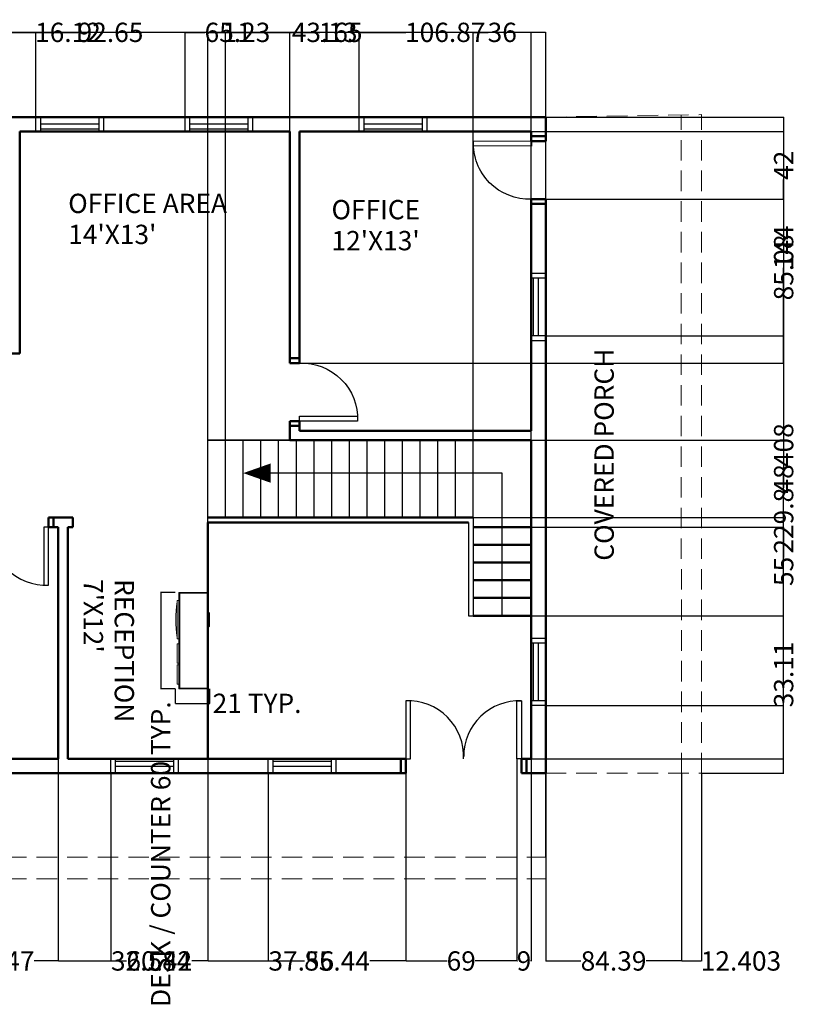
# Model space of a CAD drawing. Units: inches. Extents: x 128 to 1267, y -109 to 1208.
# Tile 4 of 8: x 784 to 1267, y -109 to 503. Entities that reach past the tile are written whole.
import ezdxf

# ---------------------------------------------------------------- set-up
doc = ezdxf.new("R2010")
doc.units = ezdxf.units.IN
doc.header["$MEASUREMENT"] = 0
doc.linetypes.add('DASHED', pattern=[19.05, 12.7, -6.35])
for name, color, linetype, lineweight in [('A-ANNO-DIMS', 2, 'Continuous', 18), ('A-AREA-IDEN', 3, 'Continuous', 25), ('A-DOOR', 4, 'Continuous', 25), ('A-FLOR-STRS', 2, 'Continuous', 25), ('A-FURN', 8, 'Continuous', 18), ('A-GLAZ', 3, 'Continuous', 25), ('A-ROOF-OVHD', 9, 'DASHED', 18), ('A-WALL', 7, 'Continuous', 50)]:
    doc.layers.add(name, color=color, linetype=linetype, lineweight=lineweight)
doc.styles.get("Standard").update_dxf_attribs({"font": 'arial.ttf'})
doc.dimstyles.get("Standard").update_dxf_attribs({"dimtxt": 12, "dimasz": 0.18, "dimexe": 0.18, "dimexo": 0.0625, "dimgap": 0.09, "dimtad": 0, "dimdec": 1, "dimzin": 0, "dimdsep": 46, "dimlunit": 3, "dimtxsty": 'Standard', "dimcen": 0.09, "dimadec": 0, "dimazin": 0, "dimtfac": 1, "dimtdec": 1, "dimtofl": 0, "dimtmove": 0, "dimatfit": 3, "dimfxl": 1, "dimtolj": 1, "dimtzin": 0, "dimarcsym": 0})

# ---------------------------------------------------------------- blocks, each defined once
blk = doc.blocks.new('Entertainment Center')
for p, q in [((-4, 0), (-5, -1)), ((4, 0), (-4, 0)), ((5, -1), (4, 0)), ((-17, -19), (-17, -1)), ((-17, -1), (43, -1)), ((-16.5, -18.5), (-16.5, -1.5)), ((-16.5, -1.5), (42.5, -1.5)), ((42.5, -1.5), (42.5, -18.5)), ((43, -1), (43, -19)), ((43, -19), (-17, -19)), ((42.5, -18.5), (-16.5, -18.5)), ((-12, -20), (-12, -19)), ((12, -20), (-12, -20)), ((12, -19), (12, -20)), ((15, -20), (15, -19)), ((27, -20), (15, -20)), ((27, -19), (27, -20)), ((28, -20), (28, -19)), ((40, -20), (28, -20)), ((40, -19), (40, -20))]:
    blk.add_line(p, q)
blk.add_arc((0, 40), 61, 259.6111, 280.3889)
blk = doc.blocks.new('DOOR-900')
blk.add_lwpolyline([(460.06, 187.64), (457.06, 187.64), (457.06, 151.64), (460.06, 151.64)], close=True)
blk.add_arc((458.56, 186.14), 34.53, 177.51045, 272.48955)
blk = doc.blocks.new('WIN-900')
for p, q in [((1102.06, 345.56), (1111.06, 345.56)), ((1102.06, 342.56), (1111.06, 342.56)), ((1103.56, 306.56), (1103.56, 342.56)), ((1106.56, 306.56), (1106.56, 342.56)), ((1111.06, 306.56), (1102.06, 306.56)), ((1111.06, 303.56), (1102.06, 303.56))]:
    blk.add_line(p, q)
blk = doc.blocks.new('*D12')
at = {"layer": 'A-ANNO-DIMS', "color": 0, "lineweight": -2, "transparency": 16777216}
for p, q in [((880.66, 147.14), (871.54, 147.14)), ((871.72, 146.96), (871.72, 87.32)), ((880.66, 87.14), (871.54, 87.14)), ((871.72, 87.14), (871.72, 86.96))]:
    blk.add_line(p, q, dxfattribs=at)
at = {"layer": 'A-ANNO-DIMS', "color": 0, "transparency": 16777216}
for points in [[(871.69, 146.96), (871.75, 146.96), (871.72, 147.14)], [(871.69, 87.32), (871.75, 87.32), (871.72, 87.14)]]:
    blk.add_solid(points, dxfattribs=at)
at = {"layer": 'Defpoints', "color": 0, "transparency": 16777216}
for p in [(880.72, 147.14), (871.72, 87.14), (880.72, 87.14)]:
    blk.add_point(p, dxfattribs=at)
at = {"layer": 'A-ANNO-DIMS', "color": 0, "transparency": 16777216, "insert": (871.72, -15.62), "char_height": 12, "attachment_point": 5, "rotation": 90}
blk.add_mtext('\\A1;DESK / COUNTER 60 TYP.', dxfattribs=at)
blk = doc.blocks.new('*D13')
at = {"layer": 'A-ANNO-DIMS', "color": 0, "lineweight": -2, "transparency": 16777216}
for p, q in [((880.72, 87.08), (880.72, 77.96)), ((902.06, 87.08), (902.06, 77.96)), ((880.9, 78.14), (901.88, 78.14)), ((902.06, 78.14), (902.24, 78.14))]:
    blk.add_line(p, q, dxfattribs=at)
at = {"layer": 'A-ANNO-DIMS', "color": 0, "transparency": 16777216}
for points in [[(880.9, 78.17), (880.9, 78.11), (880.72, 78.14)], [(901.88, 78.17), (901.88, 78.11), (902.06, 78.14)]]:
    blk.add_solid(points, dxfattribs=at)
at = {"layer": 'Defpoints', "color": 0, "transparency": 16777216}
for p in [(880.72, 87.14), (902.06, 87.14), (902.06, 78.14)]:
    blk.add_point(p, dxfattribs=at)
at = {"layer": 'A-ANNO-DIMS', "color": 0, "transparency": 16777216, "insert": (931.63, 78.14), "char_height": 12, "attachment_point": 5}
blk.add_mtext('\\A1;21 TYP.', dxfattribs=at)
blk = doc.blocks.new('*D22')
at = {"layer": 'A-ANNO-DIMS', "color": 0, "lineweight": -2, "transparency": 16777216}
for p, q in [((223.06, -17.52), (223.06, 495.44)), ((223.24, 495.26), (653.69, 495.26)), ((1110.88, 495.26), (680.42, 495.26)), ((1111.06, -17.52), (1111.06, 495.44))]:
    blk.add_line(p, q, dxfattribs=at)
at = {"layer": 'A-ANNO-DIMS', "color": 0, "transparency": 16777216}
for points in [[(223.24, 495.29), (223.24, 495.23), (223.06, 495.26)], [(1110.88, 495.29), (1110.88, 495.23), (1111.06, 495.26)]]:
    blk.add_solid(points, dxfattribs=at)
at = {"layer": 'Defpoints', "color": 0, "transparency": 16777216}
for p in [(1111.06, 495.26), (223.06, -17.58), (1111.06, -17.58)]:
    blk.add_point(p, dxfattribs=at)
at = {"layer": 'A-ANNO-DIMS', "color": 0, "transparency": 16777216, "insert": (667.06, 495.26), "char_height": 12, "attachment_point": 5}
blk.add_mtext('\\A1;888', dxfattribs=at)
blk = doc.blocks.new('*D23')
at = {"layer": 'A-ANNO-DIMS', "color": 0, "lineweight": -2, "transparency": 16777216}
for p, q in [((1111.12, 442.64), (1259.18, 442.64)), ((1259, 442.46), (1259, 252.24)), ((1259, 34.82), (1259, 225.04)), ((1207.91, 34.64), (1259.18, 34.64))]:
    blk.add_line(p, q, dxfattribs=at)
at = {"layer": 'A-ANNO-DIMS', "color": 0, "transparency": 16777216}
for points in [[(1258.97, 442.46), (1259.03, 442.46), (1259, 442.64)], [(1258.97, 34.82), (1259.03, 34.82), (1259, 34.64)]]:
    blk.add_solid(points, dxfattribs=at)
at = {"layer": 'Defpoints', "color": 0, "transparency": 16777216}
for p in [(1111.06, 442.64), (1207.85, 34.64), (1259, 34.64)]:
    blk.add_point(p, dxfattribs=at)
at = {"layer": 'A-ANNO-DIMS', "color": 0, "transparency": 16777216, "insert": (1259, 238.64), "char_height": 12, "attachment_point": 5, "rotation": 90}
blk.add_mtext('\\A1;408', dxfattribs=at)
blk = doc.blocks.new('*D24')
at = {"layer": 'A-ANNO-DIMS', "color": 0, "lineweight": -2, "transparency": 16777216}
for p, q in [((1111.06, 34.58), (1111.06, -82.19)), ((1195.45, 34.58), (1195.45, -82.19)), ((1111.24, -82.01), (1132.89, -82.01)), ((1195.27, -82.01), (1173.61, -82.01))]:
    blk.add_line(p, q, dxfattribs=at)
at = {"layer": 'A-ANNO-DIMS', "color": 0, "transparency": 16777216}
for points in [[(1111.24, -81.98), (1111.24, -82.04), (1111.06, -82.01)], [(1195.27, -81.98), (1195.27, -82.04), (1195.45, -82.01)]]:
    blk.add_solid(points, dxfattribs=at)
at = {"layer": 'Defpoints', "color": 0, "transparency": 16777216}
for p in [(1111.06, 34.64), (1195.45, 34.64), (1195.45, -82.01)]:
    blk.add_point(p, dxfattribs=at)
at = {"layer": 'A-ANNO-DIMS', "color": 0, "transparency": 16777216, "insert": (1153.25, -82.01), "char_height": 12, "attachment_point": 5}
blk.add_mtext('\\A1;84.39', dxfattribs=at)
blk = doc.blocks.new('*D25')
at = {"layer": 'A-ANNO-DIMS', "color": 0, "lineweight": -2, "transparency": 16777216}
for p, q in [((1195.45, 34.58), (1195.45, -82.19)), ((1207.85, 34.58), (1207.85, -82.19)), ((1195.63, -82.01), (1207.67, -82.01)), ((1207.85, -82.01), (1208.03, -82.01))]:
    blk.add_line(p, q, dxfattribs=at)
at = {"layer": 'A-ANNO-DIMS', "color": 0, "transparency": 16777216}
for points in [[(1195.63, -81.98), (1195.63, -82.04), (1195.45, -82.01)], [(1207.67, -81.98), (1207.67, -82.04), (1207.85, -82.01)]]:
    blk.add_solid(points, dxfattribs=at)
at = {"layer": 'Defpoints', "color": 0, "transparency": 16777216}
for p in [(1195.45, 34.64), (1207.85, 34.64), (1207.85, -82.01)]:
    blk.add_point(p, dxfattribs=at)
at = {"layer": 'A-ANNO-DIMS', "color": 0, "transparency": 16777216, "insert": (1232.46, -82.01), "char_height": 12, "attachment_point": 5}
blk.add_mtext('\\A1;12.403', dxfattribs=at)
blk = doc.blocks.new('*D35')
at = {"layer": 'A-ANNO-DIMS', "color": 0, "lineweight": -2, "transparency": 16777216}
for p, q in [((808.06, 43.58), (808.06, -82.19)), ((737.59, 34.58), (737.59, -82.19)), ((737.77, -82.01), (752.54, -82.01)), ((807.88, -82.01), (793.11, -82.01))]:
    blk.add_line(p, q, dxfattribs=at)
at = {"layer": 'A-ANNO-DIMS', "color": 0, "transparency": 16777216}
for points in [[(737.77, -81.98), (737.77, -82.04), (737.59, -82.01)], [(807.88, -81.98), (807.88, -82.04), (808.06, -82.01)]]:
    blk.add_solid(points, dxfattribs=at)
at = {"layer": 'Defpoints', "color": 0, "transparency": 16777216}
for p in [(808.06, 43.64), (737.59, 34.64), (808.06, -82.01)]:
    blk.add_point(p, dxfattribs=at)
at = {"layer": 'A-ANNO-DIMS', "color": 0, "transparency": 16777216, "insert": (772.82, -82.01), "char_height": 12, "attachment_point": 5}
blk.add_mtext('\\A1;70.47', dxfattribs=at)
blk = doc.blocks.new('*D36')
at = {"layer": 'A-ANNO-DIMS', "color": 0, "lineweight": -2, "transparency": 16777216}
for p, q in [((808.06, 43.58), (808.06, -82.19)), ((840.64, 34.58), (840.64, -82.19)), ((808.24, -82.01), (840.46, -82.01)), ((840.64, -82.01), (840.82, -82.01))]:
    blk.add_line(p, q, dxfattribs=at)
at = {"layer": 'A-ANNO-DIMS', "color": 0, "transparency": 16777216}
for points in [[(808.24, -81.98), (808.24, -82.04), (808.06, -82.01)], [(840.46, -81.98), (840.46, -82.04), (840.64, -82.01)]]:
    blk.add_solid(points, dxfattribs=at)
at = {"layer": 'Defpoints', "color": 0, "transparency": 16777216}
for p in [(808.06, 43.64), (840.64, 34.64), (840.64, -82.01)]:
    blk.add_point(p, dxfattribs=at)
at = {"layer": 'A-ANNO-DIMS', "color": 0, "transparency": 16777216, "insert": (865.79, -82.01), "char_height": 12, "attachment_point": 5}
blk.add_mtext('\\A1;32.584', dxfattribs=at)
blk = doc.blocks.new('*D37')
at = {"layer": 'A-ANNO-DIMS', "color": 0, "lineweight": -2, "transparency": 16777216}
for p, q in [((901.06, 43.58), (901.06, -82.19)), ((840.64, 34.58), (840.64, -82.19)), ((840.82, -82.01), (850.54, -82.01)), ((900.88, -82.01), (891.16, -82.01))]:
    blk.add_line(p, q, dxfattribs=at)
at = {"layer": 'A-ANNO-DIMS', "color": 0, "transparency": 16777216}
for points in [[(840.82, -81.98), (840.82, -82.04), (840.64, -82.01)], [(900.88, -81.98), (900.88, -82.04), (901.06, -82.01)]]:
    blk.add_solid(points, dxfattribs=at)
at = {"layer": 'Defpoints', "color": 0, "transparency": 16777216}
for p in [(901.06, 43.64), (840.64, 34.64), (901.06, -82.01)]:
    blk.add_point(p, dxfattribs=at)
at = {"layer": 'A-ANNO-DIMS', "color": 0, "transparency": 16777216, "insert": (870.85, -82.01), "char_height": 12, "attachment_point": 5}
blk.add_mtext('\\A1;60.42', dxfattribs=at)
blk = doc.blocks.new('*D38')
at = {"layer": 'A-ANNO-DIMS', "color": 0, "lineweight": -2, "transparency": 16777216}
for p, q in [((901.06, 43.58), (901.06, -82.19)), ((938.62, 34.58), (938.62, -82.19)), ((901.24, -82.01), (938.44, -82.01)), ((938.62, -82.01), (938.8, -82.01))]:
    blk.add_line(p, q, dxfattribs=at)
at = {"layer": 'A-ANNO-DIMS', "color": 0, "transparency": 16777216}
for points in [[(901.24, -81.98), (901.24, -82.04), (901.06, -82.01)], [(938.44, -81.98), (938.44, -82.04), (938.62, -82.01)]]:
    blk.add_solid(points, dxfattribs=at)
at = {"layer": 'Defpoints', "color": 0, "transparency": 16777216}
for p in [(901.06, 43.64), (938.62, 34.64), (938.62, -82.01)]:
    blk.add_point(p, dxfattribs=at)
at = {"layer": 'A-ANNO-DIMS', "color": 0, "transparency": 16777216, "insert": (959.13, -82.01), "char_height": 12, "attachment_point": 5}
blk.add_mtext('\\A1;37.56', dxfattribs=at)
blk = doc.blocks.new('*D39')
at = {"layer": 'A-ANNO-DIMS', "color": 0, "lineweight": -2, "transparency": 16777216}
for p, q in [((938.62, 34.58), (938.62, -82.19)), ((1024.06, 34.58), (1024.06, -82.19)), ((938.8, -82.01), (961.02, -82.01)), ((1023.88, -82.01), (1001.66, -82.01))]:
    blk.add_line(p, q, dxfattribs=at)
at = {"layer": 'A-ANNO-DIMS', "color": 0, "transparency": 16777216}
for points in [[(938.8, -81.98), (938.8, -82.04), (938.62, -82.01)], [(1023.88, -81.98), (1023.88, -82.04), (1024.06, -82.01)]]:
    blk.add_solid(points, dxfattribs=at)
at = {"layer": 'Defpoints', "color": 0, "transparency": 16777216}
for p in [(938.62, 34.64), (1024.06, 34.64), (1024.06, -82.01)]:
    blk.add_point(p, dxfattribs=at)
at = {"layer": 'A-ANNO-DIMS', "color": 0, "transparency": 16777216, "insert": (981.34, -82.01), "char_height": 12, "attachment_point": 5}
blk.add_mtext('\\A1;85.44', dxfattribs=at)
blk = doc.blocks.new('*D40')
at = {"layer": 'A-ANNO-DIMS', "color": 0, "lineweight": -2, "transparency": 16777216}
for p, q in [((1093.06, 43.58), (1093.06, -82.19)), ((1024.06, 34.58), (1024.06, -82.19)), ((1024.24, -82.01), (1049.83, -82.01)), ((1092.88, -82.01), (1067.29, -82.01))]:
    blk.add_line(p, q, dxfattribs=at)
at = {"layer": 'A-ANNO-DIMS', "color": 0, "transparency": 16777216}
for points in [[(1024.24, -81.98), (1024.24, -82.04), (1024.06, -82.01)], [(1092.88, -81.98), (1092.88, -82.04), (1093.06, -82.01)]]:
    blk.add_solid(points, dxfattribs=at)
at = {"layer": 'Defpoints', "color": 0, "transparency": 16777216}
for p in [(1093.06, 43.64), (1024.06, 34.64), (1093.06, -82.01)]:
    blk.add_point(p, dxfattribs=at)
at = {"layer": 'A-ANNO-DIMS', "color": 0, "transparency": 16777216, "insert": (1058.56, -82.01), "char_height": 12, "attachment_point": 5}
blk.add_mtext('\\A1;69', dxfattribs=at)
blk = doc.blocks.new('*D41')
at = {"layer": 'A-ANNO-DIMS', "color": 0, "lineweight": -2, "transparency": 16777216}
for p, q in [((1093.06, 43.58), (1093.06, -82.19)), ((1102.06, 43.58), (1102.06, -82.19)), ((1093.24, -82.01), (1093.52, -82.01)), ((1101.88, -82.01), (1101.59, -82.01))]:
    blk.add_line(p, q, dxfattribs=at)
at = {"layer": 'A-ANNO-DIMS', "color": 0, "transparency": 16777216}
for points in [[(1093.24, -81.98), (1093.24, -82.04), (1093.06, -82.01)], [(1101.88, -81.98), (1101.88, -82.04), (1102.06, -82.01)]]:
    blk.add_solid(points, dxfattribs=at)
at = {"layer": 'Defpoints', "color": 0, "transparency": 16777216}
for p in [(1093.06, 43.64), (1102.06, 43.64), (1102.06, -82.01)]:
    blk.add_point(p, dxfattribs=at)
at = {"layer": 'A-ANNO-DIMS', "color": 0, "transparency": 16777216, "insert": (1097.56, -82.01), "char_height": 12, "attachment_point": 5}
blk.add_mtext('\\A1;9', dxfattribs=at)
blk = doc.blocks.new('*D51')
at = {"layer": 'A-ANNO-DIMS', "color": 0, "lineweight": -2, "transparency": 16777216}
for p, q in [((778.06, 433.7), (778.06, 495.44)), ((778.24, 495.26), (794, 495.26)), ((794.18, 442.7), (794.18, 495.44)), ((794.18, 495.26), (794.36, 495.26))]:
    blk.add_line(p, q, dxfattribs=at)
at = {"layer": 'A-ANNO-DIMS', "color": 0, "transparency": 16777216}
for points in [[(778.24, 495.29), (778.24, 495.23), (778.06, 495.26)], [(794, 495.29), (794, 495.23), (794.18, 495.26)]]:
    blk.add_solid(points, dxfattribs=at)
at = {"layer": 'Defpoints', "color": 0, "transparency": 16777216}
for p in [(794.18, 495.26), (794.18, 442.64), (778.06, 433.64)]:
    blk.add_point(p, dxfattribs=at)
at = {"layer": 'A-ANNO-DIMS', "color": 0, "transparency": 16777216, "insert": (814.07, 495.26), "char_height": 12, "attachment_point": 5}
blk.add_mtext('\\A1;16.12', dxfattribs=at)
blk = doc.blocks.new('*D52')
at = {"layer": 'A-ANNO-DIMS', "color": 0, "lineweight": -2, "transparency": 16777216}
for p, q in [((794.18, 442.7), (794.18, 495.44)), ((794.36, 495.26), (820.12, 495.26)), ((886.65, 495.26), (860.88, 495.26)), ((886.83, 442.7), (886.83, 495.44))]:
    blk.add_line(p, q, dxfattribs=at)
at = {"layer": 'A-ANNO-DIMS', "color": 0, "transparency": 16777216}
for points in [[(794.36, 495.29), (794.36, 495.23), (794.18, 495.26)], [(886.65, 495.29), (886.65, 495.23), (886.83, 495.26)]]:
    blk.add_solid(points, dxfattribs=at)
at = {"layer": 'Defpoints', "color": 0, "transparency": 16777216}
for p in [(886.83, 495.26), (794.18, 442.64), (886.83, 442.64)]:
    blk.add_point(p, dxfattribs=at)
at = {"layer": 'A-ANNO-DIMS', "color": 0, "transparency": 16777216, "insert": (840.5, 495.26), "char_height": 12, "attachment_point": 5}
blk.add_mtext('\\A1;92.65', dxfattribs=at)
blk = doc.blocks.new('*D53')
at = {"layer": 'A-ANNO-DIMS', "color": 0, "lineweight": -2, "transparency": 16777216}
for p, q in [((886.83, 442.7), (886.83, 495.44)), ((887.01, 495.26), (899.07, 495.26)), ((951.88, 495.26), (939.81, 495.26)), ((952.06, 433.7), (952.06, 495.44))]:
    blk.add_line(p, q, dxfattribs=at)
at = {"layer": 'A-ANNO-DIMS', "color": 0, "transparency": 16777216}
for points in [[(887.01, 495.29), (887.01, 495.23), (886.83, 495.26)], [(951.88, 495.29), (951.88, 495.23), (952.06, 495.26)]]:
    blk.add_solid(points, dxfattribs=at)
at = {"layer": 'Defpoints', "color": 0, "transparency": 16777216}
for p in [(952.06, 495.26), (886.83, 442.64), (952.06, 433.64)]:
    blk.add_point(p, dxfattribs=at)
at = {"layer": 'A-ANNO-DIMS', "color": 0, "transparency": 16777216, "insert": (919.44, 495.26), "char_height": 12, "attachment_point": 5}
blk.add_mtext('\\A1;65.23', dxfattribs=at)
blk = doc.blocks.new('*D54')
at = {"layer": 'A-ANNO-DIMS', "color": 0, "lineweight": -2, "transparency": 16777216}
for p, q in [((952.06, 433.7), (952.06, 495.44)), ((952.24, 495.26), (953.04, 495.26)), ((995, 495.26), (994.2, 495.26)), ((995.18, 442.7), (995.18, 495.44))]:
    blk.add_line(p, q, dxfattribs=at)
at = {"layer": 'A-ANNO-DIMS', "color": 0, "transparency": 16777216}
for points in [[(952.24, 495.29), (952.24, 495.23), (952.06, 495.26)], [(995, 495.29), (995, 495.23), (995.18, 495.26)]]:
    blk.add_solid(points, dxfattribs=at)
at = {"layer": 'Defpoints', "color": 0, "transparency": 16777216}
for p in [(995.18, 495.26), (995.18, 442.64), (952.06, 433.64)]:
    blk.add_point(p, dxfattribs=at)
at = {"layer": 'A-ANNO-DIMS', "color": 0, "transparency": 16777216, "insert": (973.62, 495.26), "char_height": 12, "attachment_point": 5}
blk.add_mtext('\\A1;43.13', dxfattribs=at)
blk = doc.blocks.new('*D55')
at = {"layer": 'A-ANNO-DIMS', "color": 0, "lineweight": -2, "transparency": 16777216}
for p, q in [((995.18, 442.7), (995.18, 495.44)), ((995.36, 495.26), (1024.19, 495.26)), ((1101.88, 495.26), (1073.05, 495.26)), ((1102.06, 433.7), (1102.06, 495.44))]:
    blk.add_line(p, q, dxfattribs=at)
at = {"layer": 'A-ANNO-DIMS', "color": 0, "transparency": 16777216}
for points in [[(995.36, 495.29), (995.36, 495.23), (995.18, 495.26)], [(1101.88, 495.29), (1101.88, 495.23), (1102.06, 495.26)]]:
    blk.add_solid(points, dxfattribs=at)
at = {"layer": 'Defpoints', "color": 0, "transparency": 16777216}
for p in [(1102.06, 495.26), (995.18, 442.64), (1102.06, 433.64)]:
    blk.add_point(p, dxfattribs=at)
at = {"layer": 'A-ANNO-DIMS', "color": 0, "transparency": 16777216, "insert": (1048.62, 495.26), "char_height": 12, "attachment_point": 5}
blk.add_mtext('\\A1;106.87', dxfattribs=at)
blk = doc.blocks.new('*D60')
at = {"layer": 'A-ANNO-DIMS', "color": 0, "lineweight": -2, "transparency": 16777216}
for p, q in [((1111.12, 76.75), (1259.18, 76.75)), ((1259, 76.75), (1259, 76.93)), ((1259, 43.82), (1259, 76.57)), ((1102.12, 43.64), (1259.18, 43.64))]:
    blk.add_line(p, q, dxfattribs=at)
at = {"layer": 'A-ANNO-DIMS', "color": 0, "transparency": 16777216}
for points in [[(1258.97, 76.57), (1259.03, 76.57), (1259, 76.75)], [(1258.97, 43.82), (1259.03, 43.82), (1259, 43.64)]]:
    blk.add_solid(points, dxfattribs=at)
at = {"layer": 'Defpoints', "color": 0, "transparency": 16777216}
for p in [(1111.06, 76.75), (1259, 76.75), (1102.06, 43.64)]:
    blk.add_point(p, dxfattribs=at)
at = {"layer": 'A-ANNO-DIMS', "color": 0, "transparency": 16777216, "insert": (1259, 96.11), "char_height": 12, "attachment_point": 5, "rotation": 90}
blk.add_mtext('\\A1;33.11', dxfattribs=at)
blk = doc.blocks.new('*D61')
at = {"layer": 'A-ANNO-DIMS', "color": 0, "lineweight": -2, "transparency": 16777216}
for p, q in [((1111.12, 306.56), (1259.18, 306.56)), ((1259, 306.38), (1259, 212.11)), ((1259, 76.93), (1259, 171.21)), ((1111.12, 76.75), (1259.18, 76.75))]:
    blk.add_line(p, q, dxfattribs=at)
at = {"layer": 'A-ANNO-DIMS', "color": 0, "transparency": 16777216}
for points in [[(1258.97, 306.38), (1259.03, 306.38), (1259, 306.56)], [(1258.97, 76.93), (1259.03, 76.93), (1259, 76.75)]]:
    blk.add_solid(points, dxfattribs=at)
at = {"layer": 'Defpoints', "color": 0, "transparency": 16777216}
for p in [(1111.06, 306.56), (1259, 306.56), (1111.06, 76.75)]:
    blk.add_point(p, dxfattribs=at)
at = {"layer": 'A-ANNO-DIMS', "color": 0, "transparency": 16777216, "insert": (1259, 191.66), "char_height": 12, "attachment_point": 5, "rotation": 90}
blk.add_mtext('\\A1;229.8', dxfattribs=at)
blk = doc.blocks.new('*D62')
at = {"layer": 'A-ANNO-DIMS', "color": 0, "lineweight": -2, "transparency": 16777216}
for p, q in [((1111.12, 391.64), (1259.18, 391.64)), ((1259, 391.46), (1259, 369.46)), ((1259, 306.74), (1259, 328.74)), ((1111.12, 306.56), (1259.18, 306.56))]:
    blk.add_line(p, q, dxfattribs=at)
at = {"layer": 'A-ANNO-DIMS', "color": 0, "transparency": 16777216}
for points in [[(1258.97, 391.46), (1259.03, 391.46), (1259, 391.64)], [(1258.97, 306.74), (1259.03, 306.74), (1259, 306.56)]]:
    blk.add_solid(points, dxfattribs=at)
at = {"layer": 'Defpoints', "color": 0, "transparency": 16777216}
for p in [(1111.06, 391.64), (1259, 391.64), (1111.06, 306.56)]:
    blk.add_point(p, dxfattribs=at)
at = {"layer": 'A-ANNO-DIMS', "color": 0, "transparency": 16777216, "insert": (1259, 349.1), "char_height": 12, "attachment_point": 5, "rotation": 90}
blk.add_mtext('\\A1;85.08', dxfattribs=at)
blk = doc.blocks.new('*D63')
at = {"layer": 'A-ANNO-DIMS', "color": 0, "lineweight": -2, "transparency": 16777216}
for p, q in [((1102.12, 433.64), (1259.18, 433.64)), ((1259, 433.46), (1259, 421.5)), ((1259, 391.82), (1259, 403.78)), ((1111.12, 391.64), (1259.18, 391.64))]:
    blk.add_line(p, q, dxfattribs=at)
at = {"layer": 'A-ANNO-DIMS', "color": 0, "transparency": 16777216}
for points in [[(1258.97, 433.46), (1259.03, 433.46), (1259, 433.64)], [(1258.97, 391.82), (1259.03, 391.82), (1259, 391.64)]]:
    blk.add_solid(points, dxfattribs=at)
at = {"layer": 'Defpoints', "color": 0, "transparency": 16777216}
for p in [(1102.06, 433.64), (1259, 433.64), (1111.06, 391.64)]:
    blk.add_point(p, dxfattribs=at)
at = {"layer": 'A-ANNO-DIMS', "color": 0, "transparency": 16777216, "insert": (1259, 412.64), "char_height": 12, "attachment_point": 5, "rotation": 90}
blk.add_mtext('\\A1;42', dxfattribs=at)
blk = doc.blocks.new('*D65')
at = {"layer": 'A-ANNO-DIMS', "color": 0, "lineweight": -2, "transparency": 16777216}
for p, q in [((1066.12, 187.64), (1259.18, 187.64)), ((1259, 187.46), (1259, 168.87)), ((1259, 132.82), (1259, 151.41)), ((1066.12, 132.64), (1259.18, 132.64))]:
    blk.add_line(p, q, dxfattribs=at)
at = {"layer": 'A-ANNO-DIMS', "color": 0, "transparency": 16777216}
for points in [[(1258.97, 187.46), (1259.03, 187.46), (1259, 187.64)], [(1258.97, 132.82), (1259.03, 132.82), (1259, 132.64)]]:
    blk.add_solid(points, dxfattribs=at)
at = {"layer": 'Defpoints', "color": 0, "transparency": 16777216}
for p in [(1066.06, 187.64), (1066.06, 132.64), (1259, 132.64)]:
    blk.add_point(p, dxfattribs=at)
at = {"layer": 'A-ANNO-DIMS', "color": 0, "transparency": 16777216, "insert": (1259, 160.14), "char_height": 12, "attachment_point": 5, "rotation": 90}
blk.add_mtext('\\A1;55', dxfattribs=at)
blk = doc.blocks.new('*D88')
at = {"layer": 'A-ANNO-DIMS', "color": 0, "lineweight": -2, "transparency": 16777216}
for p, q in [((901.06, 241.7), (901.06, 495.44)), ((901.24, 495.26), (970.73, 495.26)), ((1065.88, 495.26), (996.38, 495.26)), ((1066.06, 241.7), (1066.06, 495.44))]:
    blk.add_line(p, q, dxfattribs=at)
at = {"layer": 'A-ANNO-DIMS', "color": 0, "transparency": 16777216}
for points in [[(901.24, 495.29), (901.24, 495.23), (901.06, 495.26)], [(1065.88, 495.29), (1065.88, 495.23), (1066.06, 495.26)]]:
    blk.add_solid(points, dxfattribs=at)
at = {"layer": 'Defpoints', "color": 0, "transparency": 16777216}
for p in [(1066.06, 495.26), (901.06, 241.64), (1066.06, 241.64)]:
    blk.add_point(p, dxfattribs=at)
at = {"layer": 'A-ANNO-DIMS', "color": 0, "transparency": 16777216, "insert": (983.56, 495.26), "char_height": 12, "attachment_point": 5}
blk.add_mtext('\\A1;165', dxfattribs=at)
blk = doc.blocks.new('*D89')
at = {"layer": 'A-ANNO-DIMS', "color": 0, "lineweight": -2, "transparency": 16777216}
for p, q in [((901.12, 241.64), (1259.18, 241.64)), ((1259, 241.46), (1259, 226.58)), ((1259, 193.82), (1259, 208.7)), ((901.12, 193.64), (1259.18, 193.64))]:
    blk.add_line(p, q, dxfattribs=at)
at = {"layer": 'A-ANNO-DIMS', "color": 0, "transparency": 16777216}
for points in [[(1258.97, 241.46), (1259.03, 241.46), (1259, 241.64)], [(1258.97, 193.82), (1259.03, 193.82), (1259, 193.64)]]:
    blk.add_solid(points, dxfattribs=at)
at = {"layer": 'Defpoints', "color": 0, "transparency": 16777216}
for p in [(901.06, 241.64), (901.06, 193.64), (1259, 193.64)]:
    blk.add_point(p, dxfattribs=at)
at = {"layer": 'A-ANNO-DIMS', "color": 0, "transparency": 16777216, "insert": (1259, 217.64), "char_height": 12, "attachment_point": 5, "rotation": 90}
blk.add_mtext('\\A1;48', dxfattribs=at)
blk = doc.blocks.new('*D90')
at = {"layer": 'A-ANNO-DIMS', "color": 0, "lineweight": -2, "transparency": 16777216}
for p, q in [((901.06, 241.7), (901.06, 495.44)), ((901.24, 495.26), (911.88, 495.26)), ((912.06, 241.7), (912.06, 495.44)), ((912.06, 495.26), (912.24, 495.26))]:
    blk.add_line(p, q, dxfattribs=at)
at = {"layer": 'A-ANNO-DIMS', "color": 0, "transparency": 16777216}
for points in [[(901.24, 495.29), (901.24, 495.23), (901.06, 495.26)], [(911.88, 495.29), (911.88, 495.23), (912.06, 495.26)]]:
    blk.add_solid(points, dxfattribs=at)
at = {"layer": 'Defpoints', "color": 0, "transparency": 16777216}
for p in [(912.06, 495.26), (901.06, 241.64), (912.06, 241.64)]:
    blk.add_point(p, dxfattribs=at)
at = {"layer": 'A-ANNO-DIMS', "color": 0, "transparency": 16777216, "insert": (919.2, 495.26), "char_height": 12, "attachment_point": 5}
blk.add_mtext('\\A1;11', dxfattribs=at)
blk = doc.blocks.new('*D91')
at = {"layer": 'A-ANNO-DIMS', "color": 0, "lineweight": -2, "transparency": 16777216}
for p, q in [((1066.06, 241.7), (1066.06, 495.44)), ((1066.24, 495.26), (1075.38, 495.26)), ((1101.88, 495.26), (1092.73, 495.26)), ((1102.06, 241.7), (1102.06, 495.44))]:
    blk.add_line(p, q, dxfattribs=at)
at = {"layer": 'A-ANNO-DIMS', "color": 0, "transparency": 16777216}
for points in [[(1066.24, 495.29), (1066.24, 495.23), (1066.06, 495.26)], [(1101.88, 495.29), (1101.88, 495.23), (1102.06, 495.26)]]:
    blk.add_solid(points, dxfattribs=at)
at = {"layer": 'Defpoints', "color": 0, "transparency": 16777216}
for p in [(1102.06, 495.26), (1066.06, 241.64), (1102.06, 241.64)]:
    blk.add_point(p, dxfattribs=at)
at = {"layer": 'A-ANNO-DIMS', "color": 0, "transparency": 16777216, "insert": (1084.06, 495.26), "char_height": 12, "attachment_point": 5}
blk.add_mtext('\\A1;36', dxfattribs=at)
blk = doc.blocks.new('*D92')
at = {"layer": 'A-ANNO-DIMS', "color": 0, "lineweight": -2, "transparency": 16777216}
for p, q in [((958.12, 433.64), (1259.18, 433.64)), ((1259, 433.46), (1259, 374.4)), ((1259, 289.82), (1259, 348.88)), ((958.12, 289.64), (1259.18, 289.64))]:
    blk.add_line(p, q, dxfattribs=at)
at = {"layer": 'A-ANNO-DIMS', "color": 0, "transparency": 16777216}
for points in [[(1258.97, 433.46), (1259.03, 433.46), (1259, 433.64)], [(1258.97, 289.82), (1259.03, 289.82), (1259, 289.64)]]:
    blk.add_solid(points, dxfattribs=at)
at = {"layer": 'Defpoints', "color": 0, "transparency": 16777216}
for p in [(958.06, 433.64), (1259, 433.64), (958.06, 289.64)]:
    blk.add_point(p, dxfattribs=at)
at = {"layer": 'A-ANNO-DIMS', "color": 0, "transparency": 16777216, "insert": (1259, 361.64), "char_height": 12, "attachment_point": 5, "rotation": 90}
blk.add_mtext('\\A1;144', dxfattribs=at)

msp = doc.modelspace()

# ---------------------------------------------------------------- linework, layer by layer
at = {"layer": 'A-DOOR'}
msp.add_lwpolyline([(1096.056, 43.6399), (1093.056, 43.6399), (1093.056, 79.6399), (1096.056, 79.6399)], close=True, dxfattribs=at)
msp.add_arc((1094.556, 45.2051), 34.4675, 87.5057402, 180.1083607, dxfattribs=at)
at = {"layer": 'A-FLOR-STRS'}
for p, q in [((952.056, 241.6399), (901.056, 241.6399)), ((901.056, 190.6399), (901.056, 241.6399)), ((912.056, 193.6399), (912.056, 241.6399)), ((923.056, 193.6399), (923.056, 241.6399)), ((934.056, 193.6399), (934.056, 241.6399)), ((945.056, 193.6399), (945.056, 241.6399)), ((956.056, 193.6399), (956.056, 241.6399)), ((967.056, 193.6399), (967.056, 241.6399)), ((978.056, 193.6399), (978.056, 241.6399)), ((989.056, 193.6399), (989.056, 241.6399)), ((1000.056, 193.6399), (1000.056, 241.6399)), ((1011.056, 193.6399), (1011.056, 241.6399)), ((1022.056, 193.6399), (1022.056, 241.6399)), ((1033.056, 193.6399), (1033.056, 241.6399)), ((1044.056, 193.6399), (1044.056, 241.6399)), ((1055.056, 193.6399), (1055.056, 241.6399)), ((1066.056, 193.6399), (1066.056, 241.6399)), ((1063.056, 190.6399), (1063.056, 132.6399)), ((1066.056, 193.6399), (1066.056, 187.6399)), ((1066.056, 187.6399), (1066.056, 132.6399)), ((1063.056, 132.6399), (1066.056, 132.6399))]:
    msp.add_line(p, q, dxfattribs=at)
msp.add_lwpolyline([(940.058, 221.2651, 12, 0, 0), (923.056, 221.2651, 0, 0, 0)], format="xyseb", dxfattribs=at)
msp.add_lwpolyline([(1084.056, 132.6399), (1084.056, 221.2651), (940.058, 221.2651)], dxfattribs=at)
at = {"layer": 'A-ROOF-OVHD'}
for p, q in [((1111.056, 442.6399), (1207.8491, 444.1111)), ((1195.4465, 34.6399), (1195.2782, 443.92)), ((1207.8491, 34.6399), (1207.8491, 444.1111)), ((1111.056, 34.6399), (1111.056, -23.2776)), ((1111.056, 34.6399), (1207.8491, 34.6399)), ((223.056, -17.5809), (1111.056, -17.5809)), ((223.056, -30.8598), (1111.056, -30.8598))]:
    msp.add_line(p, q, dxfattribs=at)
at = {"layer": 'A-WALL'}
for p, q in [((784.056, 295.6399), (784.056, 433.6399)), ((952.056, 433.6399), (784.056, 433.6399)), ((952.056, 295.6399), (952.056, 433.6399)), ((1102.056, 433.6399), (958.056, 433.6399)), ((958.056, 289.6399), (958.056, 433.6399)), ((1102.056, 427.6399), (1102.056, 433.6399)), ((1102.056, 430.6399), (1111.056, 430.6399)), ((1102.056, 427.6399), (1111.056, 427.6399)), ((1102.056, 259.6399), (1102.056, 391.6399)), ((1102.056, 391.6399), (1111.056, 391.6399)), ((1102.056, 388.6399), (1111.056, 388.6399)), ((784.056, 295.6399), (772.056, 295.6399)), ((952.056, 289.6399), (952.056, 295.6399)), ((958.056, 292.6399), (952.056, 292.6399)), ((958.056, 289.6399), (952.056, 289.6399)), ((1102.056, 247.6399), (1102.056, 271.6399)), ((952.056, 241.6399), (952.056, 253.6399)), ((958.056, 253.6399), (952.056, 253.6399)), ((958.056, 247.6399), (958.056, 253.6399)), ((958.056, 250.6399), (952.056, 250.6399)), ((1102.056, 247.6399), (958.056, 247.6399)), ((1102.056, 241.6399), (952.056, 241.6399)), ((1102.056, 187.6399), (1102.056, 241.6399)), ((802.056, 187.6399), (802.056, 193.6399)), ((802.056, 193.6399), (814.056, 193.6399)), ((805.056, 187.6399), (805.056, 193.6399)), ((814.056, 193.6399), (817.056, 193.6399)), ((817.056, 187.6399), (817.056, 193.6399)), ((901.056, 193.6399), (1066.056, 193.6399)), ((901.056, 190.6399), (1063.056, 190.6399)), ((901.056, 190.6399), (901.056, 43.6399)), ((802.056, 187.6399), (808.056, 187.6399)), ((808.056, 187.6399), (808.056, 43.6399)), ((814.056, 187.6399), (814.056, 43.6399)), ((814.056, 187.6399), (817.056, 187.6399)), ((1066.056, 187.6399), (1102.056, 187.6399)), ((1102.056, 43.6399), (1102.056, 187.6399)), ((1066.056, 176.6399), (1102.056, 176.6399)), ((1066.056, 165.6399), (1102.056, 165.6399)), ((1066.056, 154.6399), (1102.056, 154.6399)), ((1066.056, 143.6399), (1102.056, 143.6399)), ((1066.056, 132.6399), (1102.056, 132.6399)), ((700.056, 43.6399), (808.056, 43.6399)), ((814.056, 43.6399), (1024.056, 43.6399)), ((1021.056, 43.6399), (1021.056, 34.6399)), ((1024.056, 43.6399), (1024.056, 34.6399)), ((1096.056, 43.6399), (1096.056, 34.6399)), ((1096.056, 43.6399), (1096.056, 34.6399)), ((1096.056, 43.6399), (1102.056, 43.6399)), ((1099.056, 43.6399), (1099.056, 34.6399))]:
    msp.add_line(p, q, dxfattribs=at)
for points in [[(1111.056, 427.6399), (1111.056, 442.6399), (409.056, 442.6399)], [(1096.056, 34.6399), (1111.056, 34.6399), (1111.056, 391.6399)], [(223.056, 199.6399), (223.056, 34.6399), (1024.056, 34.6399)]]:
    msp.add_lwpolyline(points, dxfattribs=at)

# ---------------------------------------------------------------- block references
at = {"layer": 'A-DOOR', "extrusion": (0, 0, -1), "zscale": -1}
for p, rotation in [((-912.3951, -31.5689), 90.27730096420758), ((-1145.696, 713.696), 269.9999999999998)]:
    msp.add_blockref('DOOR-900', p, dxfattribs=dict(at, rotation=rotation))
at = {"layer": 'A-DOOR'}
msp.add_blockref('DOOR-900', (342, 0), dxfattribs=at)
at = {"layer": 'A-DOOR', "rotation": 180}
msp.add_blockref('DOOR-900', (1484.112, 231.2799), dxfattribs=at)
at = {"layer": 'A-FURN', "rotation": 269.9999999999477}
msp.add_blockref('Entertainment Center', (902.056, 130.1399), dxfattribs=at)
at = {"layer": 'A-GLAZ'}
for p, rotation in [((1139.7393, -668.4161), 90.00000000000024), ((1232.3909, -668.4161), 90.00000000000036), ((1340.7449, -668.4161), 90.00000000000021), ((537.0777, 1145.696), 270.0000000000005), ((635.0543, 1145.696), 270.0000000000005)]:
    msp.add_blockref('WIN-900', p, dxfattribs=dict(at, rotation=rotation))
for p in [(0, 0), (0, -226.8102)]:
    msp.add_blockref('WIN-900', p, dxfattribs=at)

# ---------------------------------------------------------------- texts
at = {"layer": 'A-AREA-IDEN'}
for s, p in [('OFFICE AREA', (814.2164, 382.9369)), ('OFFICE', (977.9075, 379.056)), ("14'X13'", (814.2164, 363.66)), ("12'X13'", (977.9075, 359.779))]:
    msp.add_text(s, height=12, dxfattribs=at).set_placement(p)
for s, rotation, p in [('COVERED PORCH', 90, (1153.406, 166.7927)), ("7'X12'", 270, (823.8349, 155.3762)), ('RECEPTION', 270, (843.1118, 155.3762))]:
    msp.add_text(s, height=12, rotation=rotation, dxfattribs=at).set_placement(p)

# ---------------------------------------------------------------- dimensions: what is measured, and where the dimension line sits
at = {"layer": 'A-ANNO-DIMS'}
for base, p1, p2, override, picture, middle in [((1111.056, 495.2611), (223.056, -17.5809), (1111.056, -17.5809), {"dimdec": 0, "dimlfac": 1, "dimrnd": 0, "dimzin": 0, "dimdsep": 46, "dimlunit": 2}, '*D22', (667.056, 495.2611)), ((794.177, 495.2611), (778.056, 433.6399), (794.177, 442.6399), {"dimdec": 2, "dimlfac": 1, "dimrnd": 0, "dimzin": 0, "dimdsep": 46, "dimlunit": 2}, '*D51', (814.0677, 495.2611)), ((886.8286, 495.2611), (794.177, 442.6399), (886.8286, 442.6399), {"dimdec": 2, "dimlfac": 1, "dimrnd": 0, "dimzin": 0, "dimdsep": 46, "dimlunit": 2}, '*D52', (840.5028, 495.2611)), ((952.056, 495.2611), (886.8286, 442.6399), (952.056, 433.6399), {"dimdec": 2, "dimlfac": 1, "dimrnd": 0, "dimzin": 0, "dimdsep": 46, "dimlunit": 2}, '*D53', (919.4423, 495.2611)), ((1066.056, 495.2611), (901.056, 241.6399), (1066.056, 241.6399), {"dimdec": 0, "dimlfac": 1, "dimrnd": 0, "dimzin": 0, "dimdsep": 46, "dimlunit": 2}, '*D88', (983.556, 495.2611)), ((912.056, 495.2611), (901.056, 241.6399), (912.056, 241.6399), {"dimdec": 0, "dimlfac": 1, "dimrnd": 0, "dimzin": 0, "dimdsep": 46, "dimlunit": 2}, '*D90', (919.1978, 495.2611)), ((995.1826, 495.2611), (952.056, 433.6399), (995.1826, 442.6399), {"dimdec": 2, "dimlfac": 1, "dimrnd": 0, "dimzin": 0, "dimdsep": 46, "dimlunit": 2}, '*D54', (973.6193, 495.2611)), ((1102.056, 495.2611), (995.1826, 442.6399), (1102.056, 433.6399), {"dimdec": 2, "dimlfac": 1, "dimrnd": 0, "dimzin": 0, "dimdsep": 46, "dimlunit": 2}, '*D55', (1048.6193, 495.2611)), ((1102.056, 495.2611), (1066.056, 241.6399), (1102.056, 241.6399), {"dimdec": 0, "dimlfac": 1, "dimrnd": 0, "dimzin": 0, "dimdsep": 46, "dimlunit": 2}, '*D91', (1084.056, 495.2611)), ((808.056, -82.0098), (737.59, 34.6399), (808.056, 43.6399), {"dimdec": 2, "dimlfac": 1, "dimrnd": 0, "dimzin": 0, "dimdsep": 46, "dimlunit": 2}, '*D35', (772.823, -82.0098)), ((840.64, -82.0098), (808.056, 43.6399), (840.64, 34.6399), {"dimdec": 3, "dimlfac": 1, "dimrnd": 0, "dimzin": 0, "dimdsep": 46, "dimlunit": 2}, '*D36', (865.79, -82.0098)), ((901.056, -82.0098), (840.64, 34.6399), (901.056, 43.6399), {"dimdec": 2, "dimlfac": 1, "dimrnd": 0, "dimzin": 0, "dimdsep": 46, "dimlunit": 2}, '*D37', (870.848, -82.0098)), ((938.6166, -82.0098), (901.056, 43.6399), (938.6166, 34.6399), {"dimdec": 2, "dimlfac": 1, "dimrnd": 0, "dimzin": 0, "dimdsep": 46, "dimlunit": 2}, '*D38', (959.1253, -82.0098)), ((1093.056, -82.0098), (1024.056, 34.6399), (1093.056, 43.6399), {"dimdec": 0, "dimlfac": 1, "dimrnd": 0, "dimzin": 0, "dimdsep": 46, "dimlunit": 2}, '*D40', (1058.556, -82.0098)), ((1102.056, -82.0098), (1093.056, 43.6399), (1102.056, 43.6399), {"dimdec": 0, "dimlfac": 1, "dimrnd": 0, "dimzin": 0, "dimdsep": 46, "dimlunit": 2}, '*D41', (1097.556, -82.0098)), ((1024.056, -82.0098), (938.6166, 34.6399), (1024.056, 34.6399), {"dimdec": 2, "dimlfac": 1, "dimrnd": 0, "dimzin": 0, "dimdsep": 46, "dimlunit": 2}, '*D39', (981.3363, -82.0098)), ((1195.4465, -82.0098), (1111.056, 34.6399), (1195.4465, 34.6399), {"dimdec": 2, "dimlfac": 1, "dimrnd": 0, "dimzin": 0, "dimdsep": 46, "dimlunit": 2}, '*D24', (1153.2513, -82.0098)), ((1207.8491, -82.0098), (1195.4465, 34.6399), (1207.8491, 34.6399), {"dimdec": 3, "dimlfac": 1, "dimrnd": 0, "dimzin": 0, "dimdsep": 46, "dimlunit": 2}, '*D25', (1232.4629, -82.0098))]:
    dim = msp.add_linear_dim(base=base, p1=p1, p2=p2, dimstyle='Standard', override=override, dxfattribs=at)
    dim.commit()
    dim.dimension.update_dxf_attribs({"geometry": picture, "text_midpoint": middle})
for base, p1, p2, override, picture, middle in [((1258.9991, 34.6399), (1111.056, 442.6399), (1207.8491, 34.6399), {"dimdec": 0, "dimlfac": 1, "dimrnd": 0, "dimzin": 0, "dimdsep": 46, "dimlunit": 2}, '*D23', (1258.9991, 238.6399)), ((1258.9991, 433.6399), (958.056, 289.6399), (958.056, 433.6399), {"dimdec": 0, "dimlfac": 1, "dimrnd": 0, "dimzin": 0, "dimdsep": 46, "dimlunit": 2}, '*D92', (1258.9991, 361.6399)), ((1258.9991, 433.6399), (1111.056, 391.6399), (1102.056, 433.6399), {"dimdec": 0, "dimlfac": 1, "dimrnd": 0, "dimzin": 0, "dimdsep": 46, "dimlunit": 2}, '*D63', (1258.9991, 412.6399)), ((1258.9991, 391.6399), (1111.056, 306.5623), (1111.056, 391.6399), {"dimdec": 2, "dimlfac": 1, "dimrnd": 0, "dimzin": 0, "dimdsep": 46, "dimlunit": 2}, '*D62', (1258.9991, 349.1011)), ((1258.9991, 306.5623), (1111.056, 76.7521), (1111.056, 306.5623), {"dimdec": 1, "dimlfac": 1, "dimrnd": 0, "dimzin": 0, "dimdsep": 46, "dimlunit": 2}, '*D61', (1258.9991, 191.6572)), ((1258.9991, 193.6399), (901.056, 241.6399), (901.056, 193.6399), {"dimdec": 0, "dimlfac": 1, "dimrnd": 0, "dimzin": 0, "dimdsep": 46, "dimlunit": 2}, '*D89', (1258.9991, 217.6399)), ((1258.9991, 132.6399), (1066.056, 187.6399), (1066.056, 132.6399), {"dimdec": 0, "dimlfac": 1, "dimrnd": 0, "dimzin": 0, "dimdsep": 46, "dimlunit": 2}, '*D65', (1258.9991, 160.1399)), ((1258.9991, 76.7521), (1102.056, 43.6399), (1111.056, 76.7521), {"dimdec": 2, "dimlfac": 1, "dimrnd": 0, "dimzin": 0, "dimdsep": 46, "dimlunit": 2}, '*D60', (1258.9991, 96.1067))]:
    dim = msp.add_linear_dim(base=base, p1=p1, p2=p2, angle=90, dimstyle='Standard', override=override, dxfattribs=at)
    dim.commit()
    dim.dimension.update_dxf_attribs({"geometry": picture, "text_midpoint": middle})
dim = msp.add_linear_dim(base=(871.7227, 87.1399), p1=(880.7227, 147.1399), p2=(880.7227, 87.1399), angle=270, text='DESK / COUNTER <> TYP.', dimstyle='Standard', override={"dimdec": 0, "dimrnd": 0, "dimzin": 0, "dimlunit": 2}, dxfattribs=at)
dim.commit()
dim.dimension.update_dxf_attribs({"geometry": '*D12', "text_midpoint": (871.7227, -15.6212)})
dim = msp.add_linear_dim(base=(902.056, 78.1399), p1=(880.7227, 87.1399), p2=(902.056, 87.1399), text='<> TYP.', dimstyle='Standard', override={"dimdec": 0, "dimrnd": 0, "dimzin": 0, "dimlunit": 2}, dxfattribs=at)
dim.commit()
dim.dimension.update_dxf_attribs({"geometry": '*D13', "text_midpoint": (931.6343, 78.1399)})

doc.saveas('drawing.dxf')
